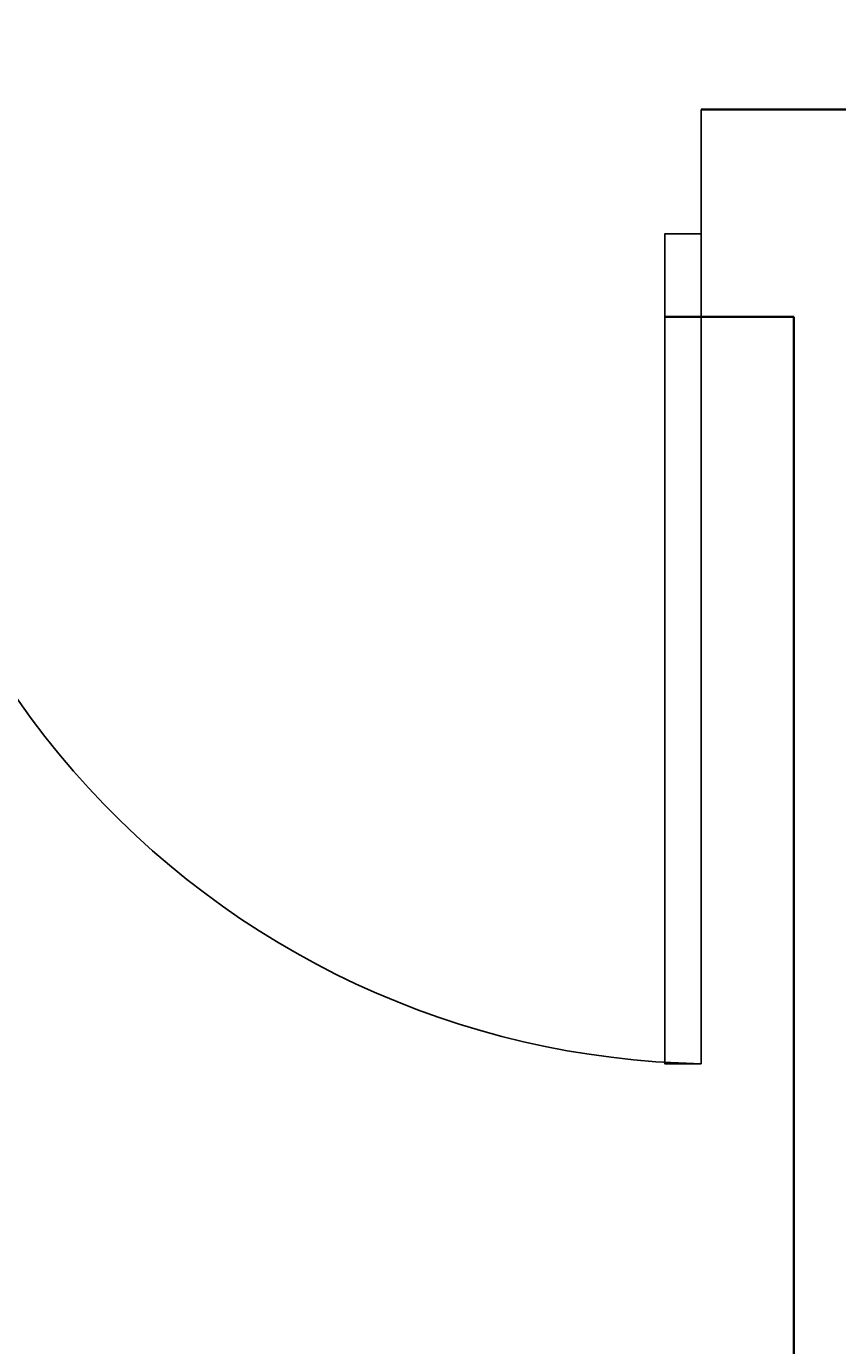
# Model space of a CAD drawing. Units: inches. Extents: x -61 to 1599, y -1316 to 257.
# Tile 89 of 204: x 298 to 321, y -318 to -280. Entities that reach past the tile are written whole.
import ezdxf

# ---------------------------------------------------------------- set-up
doc = ezdxf.new("R2010")
doc.units = ezdxf.units.IN
doc.header["$MEASUREMENT"] = 0
doc.linetypes.add('ACAD_ISO02W100', pattern=[15, 12, -3])
for name, color, linetype, lineweight in [('A-ANNO-DIMS', 2, 'Continuous', 18), ('A-WALL-JAMB', 4, 'ACAD_ISO02W100', 25), ('DOORS', 2, 'Continuous', 25), ('WALLS', 4, 'Continuous', 35)]:
    doc.layers.add(name, color=color, linetype=linetype, lineweight=lineweight)
doc.styles.get("Standard").update_dxf_attribs({"font": 'arial.ttf'})
doc.dimstyles.get("Standard").update_dxf_attribs({"dimtxt": 0.18, "dimasz": 0.18, "dimexe": 0.18, "dimexo": 0.0625, "dimgap": 0.09, "dimtad": 0, "dimtih": 1, "dimtoh": 1, "dimdec": 0, "dimzin": 0, "dimdsep": 46, "dimlunit": 3, "dimtxsty": 'Standard', "dimcen": 0.09, "dimadec": 0, "dimazin": 0, "dimtfac": 1, "dimtdec": 0, "dimtofl": 0, "dimtmove": 0, "dimatfit": 3, "dimfxl": 1, "dimtolj": 1, "dimtzin": 0, "dimarcsym": 0})

# ---------------------------------------------------------------- blocks, each defined once
blk = doc.blocks.new('DOOR-SWING-24')
blk.add_line((0, 0), (0, 3.6))
blk.add_lwpolyline([(0, 0), (0, -24), (1.05, -24), (1.05, 0)], close=True)
blk.add_arc((-0.441, 0.618), 24.622, 271.0259, 6.9559)
blk = doc.blocks.new('*D687')
at = {"layer": 'A-ANNO-DIMS', "color": 0, "lineweight": -2, "transparency": 16777216}
for p, q in [((289.418, 181.677), (-61.077, 181.677)), ((-60.897, 181.497), (-60.897, -528.952)), ((-60.897, -1239.765), (-60.897, -529.316)), ((319.64, -1239.945), (-61.077, -1239.945))]:
    blk.add_line(p, q, dxfattribs=at)
at = {"layer": 'A-ANNO-DIMS', "color": 0, "transparency": 16777216}
for points in [[(-60.927, 181.497), (-60.867, 181.497), (-60.897, 181.677)], [(-60.927, -1239.765), (-60.867, -1239.765), (-60.897, -1239.945)]]:
    blk.add_solid(points, dxfattribs=at)
at = {"layer": 'DEFPOINTS', "color": 0, "transparency": 16777216}
for p in [(289.481, 181.677), (-60.897, -1239.945), (319.703, -1239.945)]:
    blk.add_point(p, dxfattribs=at)
at = {"layer": 'A-ANNO-DIMS', "color": 0, "transparency": 16777216, "insert": (-60.897, -529.134), "char_height": 0.18, "attachment_point": 5}
blk.add_mtext('\\A1;1421.6', dxfattribs=at)
blk = doc.blocks.new('*D699')
at = {"layer": 'A-ANNO-DIMS', "color": 0, "lineweight": -2, "transparency": 16777216}
for p, q in [((835.64, -167.169), (-61.077, -167.169)), ((-60.897, -167.349), (-60.897, -306.726)), ((-60.897, -446.466), (-60.897, -307.09)), ((841.64, -446.646), (-61.077, -446.646))]:
    blk.add_line(p, q, dxfattribs=at)
at = {"layer": 'A-ANNO-DIMS', "color": 0, "transparency": 16777216}
for points in [[(-60.927, -167.349), (-60.867, -167.349), (-60.897, -167.169)], [(-60.927, -446.466), (-60.867, -446.466), (-60.897, -446.646)]]:
    blk.add_solid(points, dxfattribs=at)
at = {"layer": 'DEFPOINTS', "color": 0, "transparency": 16777216}
for p in [(835.703, -167.169), (-60.897, -446.646), (841.703, -446.646)]:
    blk.add_point(p, dxfattribs=at)
at = {"layer": 'A-ANNO-DIMS', "color": 0, "transparency": 16777216, "insert": (-60.897, -306.908), "char_height": 0.18, "attachment_point": 5}
blk.add_mtext('\\A1;279.5', dxfattribs=at)
blk = doc.blocks.new('*D702')
at = {"layer": 'A-ANNO-DIMS', "color": 0, "lineweight": -2, "transparency": 16777216}
for p, q in [((276.882, -616.882), (276.882, 257.457)), ((277.062, 257.277), (312.209, 257.277)), ((348.14, 257.277), (312.994, 257.277)), ((348.32, -616.882), (348.32, 257.457))]:
    blk.add_line(p, q, dxfattribs=at)
at = {"layer": 'A-ANNO-DIMS', "color": 0, "transparency": 16777216}
for points in [[(277.062, 257.307), (277.062, 257.247), (276.882, 257.277)], [(348.14, 257.307), (348.14, 257.247), (348.32, 257.277)]]:
    blk.add_solid(points, dxfattribs=at)
at = {"layer": 'DEFPOINTS', "color": 0, "transparency": 16777216}
for p in [(348.32, 257.277), (276.882, -616.945), (348.32, -616.945)]:
    blk.add_point(p, dxfattribs=at)
at = {"layer": 'A-ANNO-DIMS', "color": 0, "transparency": 16777216, "insert": (312.601, 257.277), "char_height": 0.18, "attachment_point": 5}
blk.add_mtext('\\A1;71.44', dxfattribs=at)

msp = doc.modelspace()

# ---------------------------------------------------------------- linework, layer by layer
at = {"layer": 'A-WALL-JAMB'}
msp.add_line((317.017, -282.3229), (317.017, -288.3229), dxfattribs=at)
at = {"layer": 'WALLS'}
for p, q in [((317.017, -282.3229), (325.7028, -282.3229)), ((315.967, -288.3229), (319.7028, -288.3229)), ((319.7028, -288.3229), (319.7028, -367.3229))]:
    msp.add_line(p, q, dxfattribs=at)

# ---------------------------------------------------------------- block references
at = {"layer": 'DOORS', "extrusion": (0, 0, -1), "zscale": -1}
msp.add_blockref('DOOR-SWING-24', (-317.017, -285.9229), dxfattribs=at)

# ---------------------------------------------------------------- dimensions: what is measured, and where the dimension line sits
at = {"layer": 'A-ANNO-DIMS'}
dim = msp.add_linear_dim(base=(348.3201, 257.2771), p1=(276.8825, -616.9446), p2=(348.3201, -616.9446), dimstyle='Standard', override={"dimdec": 2, "dimlfac": 1, "dimrnd": 0, "dimzin": 0, "dimdsep": 46, "dimlunit": 2}, dxfattribs=at)
dim.commit()
dim.dimension.update_dxf_attribs({"geometry": '*D702', "text_midpoint": (312.6013, 257.2771)})
for base, p1, p2, picture, middle in [((-60.8972, -1239.9446), (289.4807, 181.6771), (319.7028, -1239.9446), '*D687', (-60.8972, -529.1337)), ((-60.8972, -446.6462), (835.7028, -167.169), (841.7028, -446.6462), '*D699', (-60.8972, -306.9076))]:
    dim = msp.add_linear_dim(base=base, p1=p1, p2=p2, angle=90, dimstyle='Standard', override={"dimdec": 1, "dimlfac": 1, "dimrnd": 0, "dimzin": 0, "dimdsep": 46, "dimlunit": 2}, dxfattribs=at)
    dim.commit()
    dim.dimension.update_dxf_attribs({"geometry": picture, "text_midpoint": middle})

doc.saveas('drawing.dxf')
